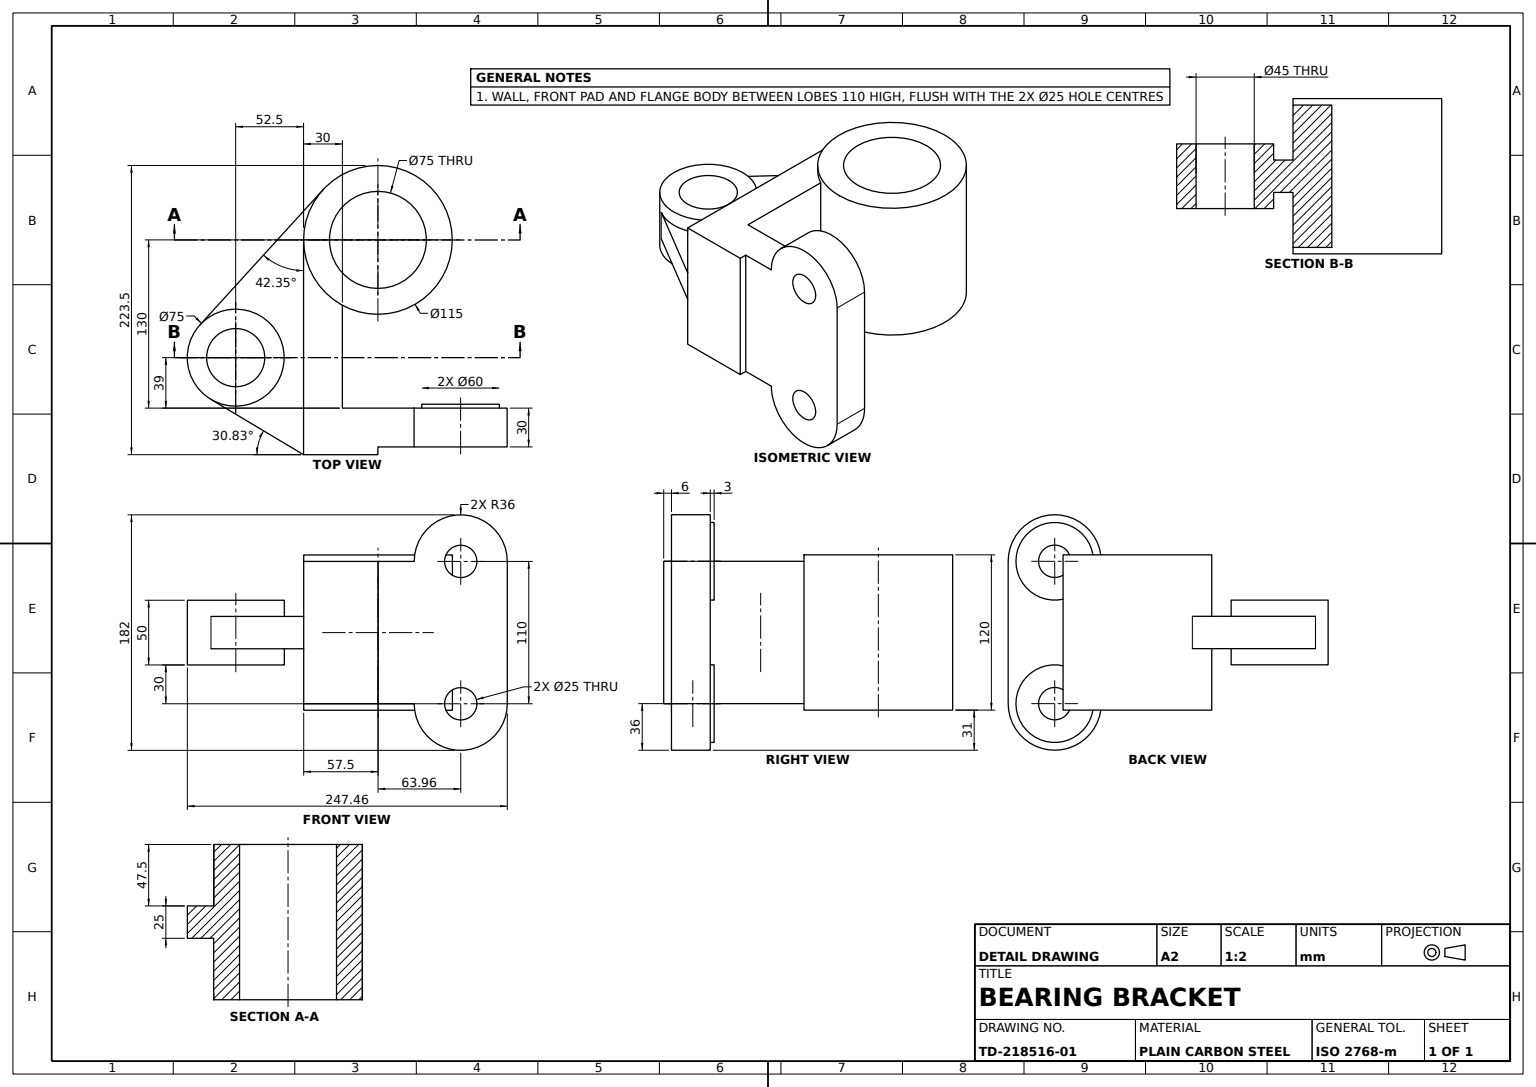
from build123d import *

# Parameters (mm, degrees)
BASE_PROFILE_SKETCH_R    = 12.5
BASE_BODY_DEPTH          = 36
SLOT_CUT_DEPTH           = 118
ARM_PROFILE_SKETCH_R     = 57.5
ARM_PROFILE_SKETCH_R_2   = 37.5
ARM_BOSS_DEPTH           = 60
ARM_BOSS_REGION_2_DEPTH  = 55
HUB_SKETCH_R             = 37.5
HUB_SKETCH_R_2           = 22.5
HUB_BOSS_DEPTH           = 25
SUPPORT_WEB_DEPTH        = 12.5
PAD_SKETCH_60X60_R       = 30
PAD_SKETCH_60X60_R_2     = 12.5
MOUNTING_PAD_60X60_DEPTH = 3


with BuildPart() as part:
    # Base Profile Sketch → Base Body (new body)
    with BuildSketch(Plane.XY):
        with BuildLine():
            Line((-66.25, 55), (19.208333333, 55))
            ThreePointArc((19.208333333, 55), (55.208333333, 91), (91.208333333, 55))
            Line((91.208333333, 55), (91.208333333, -55))
            ThreePointArc((91.208333333, -55), (55.208333333, -91), (19.208333333, -55))
            Line((19.208333333, -55), (-66.25, -55))
            Line((-66.25, -55), (-66.25, 55))
        make_face()
        with Locations((55.208333333, 55)):
            Circle(BASE_PROFILE_SKETCH_R, mode=Mode.SUBTRACT)
        with Locations((55.208333333, -55)):
            Circle(BASE_PROFILE_SKETCH_R, mode=Mode.SUBTRACT)
    extrude(amount=BASE_BODY_DEPTH)

    # Slot Sketch → Slot Cut (cut, symmetric)
    with BuildSketch(Plane(origin=(0, 0, 0), x_dir=(1, 0, 0), z_dir=(0, 1, 0))):
        Polygon((-8.75, -36), (-8.75, -30), (91.208333333, -30), (91.208333333, -36), (19.208333333, -36), align=None)
    extrude(amount=SLOT_CUT_DEPTH, both=True, mode=Mode.SUBTRACT)



with BuildPart() as body_2:
    # Arm Profile Sketch → Arm Boss (new, symmetric)
    with BuildSketch(Plane(origin=(0, 0, 0), x_dir=(1, 0, 0), z_dir=(0, 1, 0))):
        with Locations(Location((-8.75, 130, 0), (0, 0, 270))):
            Circle(ARM_PROFILE_SKETCH_R)
        with Locations(Location((-8.75, 130, 0), (0, 0, 270))):
            Circle(ARM_PROFILE_SKETCH_R_2, mode=Mode.SUBTRACT)
    extrude(amount=ARM_BOSS_DEPTH, both=True)


with BuildPart() as part_1:
    add(part.part)

    add(body_2.part)  # Arm Boss Region 2 merges body 2
    # Sketch4_3 → Arm Boss Region 2 (add, symmetric)
    with BuildSketch(Plane(origin=(0, 0, 0), x_dir=(1, 0, 0), z_dir=(0, 1, 0))):
        with BuildLine():
            Line((-66.25, 130), (-66.25, 0))
            Line((-66.25, 0), (-36.25, 0))
            Line((-36.25, 0), (-36.25, 79.502475308))
            ThreePointArc((-36.25, 79.502475308), (-58.184299833, 100.631649689), (-66.25, 130))
        make_face()
    extrude(amount=ARM_BOSS_REGION_2_DEPTH, both=True)



with BuildPart() as body_2_2:
    # Hub Sketch → Hub Boss (new, symmetric)
    with BuildSketch(Plane(origin=(0, 0, 0), x_dir=(1, 0, 0), z_dir=(0, 1, 0))):
        with Locations(Location((-118.75, 39, 0), (0, 0, 270))):
            Circle(HUB_SKETCH_R)
        with Locations(Location((-118.75, 39, 0), (0, 0, 270))):
            Circle(HUB_SKETCH_R_2, mode=Mode.SUBTRACT)
    extrude(amount=HUB_BOSS_DEPTH, both=True)


with BuildPart() as part_2:
    add(part_1.part)

    add(body_2_2.part)  # Support Web merges body 2 2
    # Web Sketch → Support Web (add, symmetric)
    with BuildSketch(Plane(origin=(0, 0, 0), x_dir=(1, 0, 0), z_dir=(0, 1, 0))):
        with BuildLine():
            Line((-146.465572764, 64.260582462), (-51.247211572, 168.732893109))
            ThreePointArc((-51.247211572, 168.732893109), (-62.368278905, 150.768489769), (-66.25, 130))
            Line((-66.25, 130), (-66.25, -36))
            Line((-66.25, -36), (-137.966934712, 6.798145701))
            ThreePointArc((-137.966934712, 6.798145701), (-81.653531514, 44.486531314), (-146.465572764, 64.260582462))
        make_face()
    extrude(amount=SUPPORT_WEB_DEPTH, both=True)

    # Pad Sketch 60x60 → Mounting Pad 60x60 (add, symmetric)
    # profile 1 of 2: a face of its own
    with BuildSketch(Plane(origin=(0, 0, 0), x_dir=(-1, 0, 0), z_dir=(0, 0, -1))):
        with Locations(Location((-55.208333333, 55, 0), (0, 0, 180))):
            Circle(PAD_SKETCH_60X60_R)
        with Locations((-55.208333333, 55)):
            Circle(PAD_SKETCH_60X60_R_2, mode=Mode.SUBTRACT)
    # profile 2 of 2: a face of its own
    with BuildSketch(Plane(origin=(0, 0, 0), x_dir=(-1, 0, 0), z_dir=(0, 0, -1))):
        with Locations(Location((-55.208333333, -55, 0), (0, 0, 180))):
            Circle(PAD_SKETCH_60X60_R)
        with Locations((-55.208333333, -55)):
            Circle(PAD_SKETCH_60X60_R_2, mode=Mode.SUBTRACT)
    extrude(amount=MOUNTING_PAD_60X60_DEPTH, both=True)


solid = part_2.part
